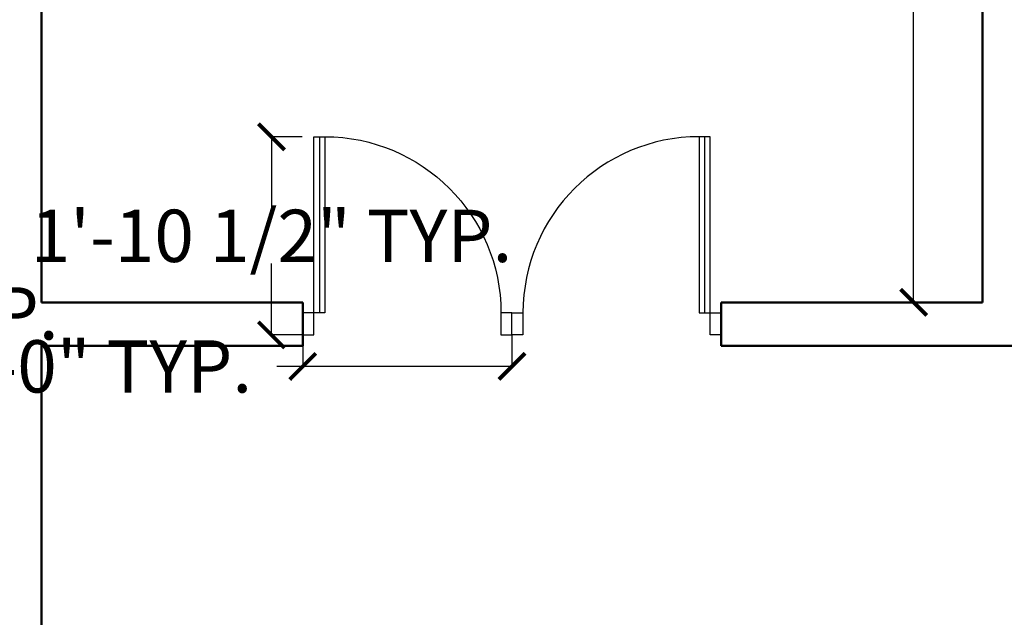
# Model space of a CAD drawing. Units: inches. Extents: x 147 to 1638, y 107 to 941.
# Tile 2 of 17: x 356 to 469, y 216 to 284. Entities that reach past the tile are written whole.
import ezdxf

# ---------------------------------------------------------------- set-up
doc = ezdxf.new("R2010")
doc.units = ezdxf.units.IN
doc.header["$MEASUREMENT"] = 0
for name, color, linetype, lineweight in [('A-ANNO-DIMS', 2, 'Continuous', 15), ('A-Door', 150, 'Continuous', 25), ('walls', 7, 'Continuous', 50)]:
    doc.layers.add(name, color=color, linetype=linetype, lineweight=lineweight)
doc.layers.add('A-Glaz', color=92, linetype='Continuous')
doc.layers.add('NT', color=1, linetype='Continuous')
doc.styles.get("Standard").update_dxf_attribs({"font": 'arial.ttf'})
doc.dimstyles.get("Standard").update_dxf_attribs({"dimtxt": 6, "dimasz": 3, "dimexe": 0.18, "dimexo": 0.0625, "dimgap": 0.09, "dimtad": 0, "dimtih": 1, "dimtoh": 1, "dimdec": 1, "dimzin": 0, "dimdsep": 46, "dimlunit": 3, "dimtxsty": 'Standard', "dimblk": 'ARCHTICK', "dimcen": 0.09, "dimadec": 0, "dimazin": 0, "dimtfac": 1, "dimtdec": 1, "dimtofl": 0, "dimtmove": 0, "dimatfit": 3, "dimfxl": 1, "dimtolj": 1, "dimtzin": 0, "dimarcsym": 0})

# ---------------------------------------------------------------- blocks, each defined once
blk = doc.blocks.new('A$C087A3AA9')
at = {"layer": 'A-Door'}
for points in [[(852.6, 94.7), (852.6, 852.6), (805.3, 852.6), (805.3, 94.7)], [(47.4, 94.7), (47.4, 0), (0, 0), (0, 94.7)], [(900, 94.7), (900, 0), (852.6, 0), (852.6, 94.7)]]:
    blk.add_lwpolyline(points, close=True, dxfattribs=at)
at = {"layer": 'A-Glaz'}
blk.add_line((828.9, 852.6), (828.9, 94.7), dxfattribs=at)
at = {"layer": 'NT'}
blk.add_arc((805.3, 94.7), 757.9, 90, 180, dxfattribs=at)
blk = doc.blocks.new('_ArchTick')
at = {"color": 0, "linetype": 'ByBlock', "const_width": 0.15}
blk.add_lwpolyline([(-0.5, -0.5), (0.5, 0.5)], dxfattribs=at)
blk = doc.blocks.new('*D30')
at = {"layer": 'A-ANNO-DIMS', "color": 0, "lineweight": -2, "transparency": 16777216}
for p, q in [((460.3, 395.72), (458.86, 395.72)), ((459.04, 395.72), (459.04, 326.82)), ((459.04, 251.72), (459.04, 320.62)), ((460.3, 251.72), (458.86, 251.72))]:
    blk.add_line(p, q, dxfattribs=at)
at = {"layer": 'Defpoints', "color": 0, "lineweight": -2, "transparency": 16777216}
for p in [(460.36, 395.72), (459.04, 251.72), (460.36, 251.72)]:
    blk.add_point(p, dxfattribs=at)
at = {"layer": 'A-ANNO-DIMS', "color": 0, "lineweight": -2, "transparency": 16777216, "xscale": 3, "yscale": 3, "zscale": 3}
for p, rotation in [((459.04, 395.72), 90), ((459.04, 251.72), 270)]:
    blk.add_blockref('_ArchTick', p, dxfattribs=dict(at, rotation=rotation))
at = {"layer": 'A-ANNO-DIMS', "color": 0, "transparency": 16777216, "insert": (459.04, 323.72), "char_height": 6, "attachment_point": 5}
blk.add_mtext("\\A1;12'", dxfattribs=at)
blk = doc.blocks.new('*D98')
at = {"layer": 'A-ANNO-DIMS', "color": 0, "lineweight": -2, "transparency": 16777216}
for p, q in [((388.94, 247.92), (388.94, 244.2)), ((412.94, 247.92), (412.94, 244.2)), ((388.94, 244.38), (385.94, 244.38)), ((412.94, 244.38), (388.94, 244.38))]:
    blk.add_line(p, q, dxfattribs=at)
at = {"layer": 'Defpoints', "color": 0, "lineweight": -2, "transparency": 16777216}
for p in [(388.94, 247.98), (412.94, 247.98), (388.94, 244.38)]:
    blk.add_point(p, dxfattribs=at)
at = {"layer": 'A-ANNO-DIMS', "color": 0, "lineweight": -2, "transparency": 16777216, "xscale": 3, "yscale": 3, "zscale": 3, "rotation": 180}
blk.add_blockref('_ArchTick', (388.94, 244.38), dxfattribs=at)
at = {"layer": 'A-ANNO-DIMS', "color": 0, "lineweight": -2, "transparency": 16777216, "xscale": 3, "yscale": 3, "zscale": 3}
blk.add_blockref('_ArchTick', (412.94, 244.38), dxfattribs=at)
at = {"layer": 'A-ANNO-DIMS', "color": 0, "transparency": 16777216, "insert": (338.48, 244.38), "char_height": 6, "attachment_point": 5}
blk.add_mtext('\\A1;SWING DOOR 2\'-0" TYP.', dxfattribs=at)
blk = doc.blocks.new('*D99')
at = {"layer": 'A-ANNO-DIMS', "color": 0, "lineweight": -2, "transparency": 16777216}
for p, q in [((388.88, 270.72), (385.16, 270.72)), ((385.34, 270.72), (385.34, 262.54)), ((385.34, 247.98), (385.34, 256.16)), ((388.88, 247.98), (385.16, 247.98))]:
    blk.add_line(p, q, dxfattribs=at)
at = {"layer": 'Defpoints', "color": 0, "lineweight": -2, "transparency": 16777216}
for p in [(385.34, 270.72), (388.94, 270.72), (388.94, 247.98)]:
    blk.add_point(p, dxfattribs=at)
at = {"layer": 'A-ANNO-DIMS', "color": 0, "lineweight": -2, "transparency": 16777216, "xscale": 3, "yscale": 3, "zscale": 3}
for p, rotation in [((385.34, 270.72), 90), ((385.34, 247.98), 270)]:
    blk.add_blockref('_ArchTick', p, dxfattribs=dict(at, rotation=rotation))
at = {"layer": 'A-ANNO-DIMS', "color": 0, "transparency": 16777216, "insert": (385.34, 259.35), "char_height": 6, "attachment_point": 5}
blk.add_mtext('\\A1;1\'-10 1/2" TYP.', dxfattribs=at)
blk = doc.blocks.new('*D111')
at = {"layer": 'A-ANNO-DIMS', "color": 0, "lineweight": -2, "transparency": 16777216}
for p, q in [((323.17, 280.75), (335.72, 280.75)), ((335.54, 280.75), (335.54, 253.66)), ((335.54, 220.18), (335.54, 247.27)), ((323.17, 220.18), (335.72, 220.18))]:
    blk.add_line(p, q, dxfattribs=at)
at = {"layer": 'Defpoints', "color": 0, "lineweight": -2, "transparency": 16777216}
for p in [(323.11, 280.75), (323.11, 220.18), (335.54, 220.18)]:
    blk.add_point(p, dxfattribs=at)
at = {"layer": 'A-ANNO-DIMS', "color": 0, "lineweight": -2, "transparency": 16777216, "xscale": 3, "yscale": 3, "zscale": 3}
for p, rotation in [((335.54, 280.75), 90), ((335.54, 220.18), 270)]:
    blk.add_blockref('_ArchTick', p, dxfattribs=dict(at, rotation=rotation))
at = {"layer": 'A-ANNO-DIMS', "color": 0, "transparency": 16777216, "insert": (335.54, 250.46), "char_height": 6, "attachment_point": 5}
blk.add_mtext('\\A1;5\'-0 1/2" TYP.', dxfattribs=at)

msp = doc.modelspace()

# ---------------------------------------------------------------- linework, layer by layer
at = {"layer": 'walls'}
for p, q in [((358.94, 395.72), (358.94, 251.72)), ((466.94, 395.72), (466.94, 251.72)), ((358.94, 251.72), (388.94, 251.72)), ((388.94, 246.72), (388.94, 251.72)), ((436.94, 246.72), (436.94, 251.72)), ((436.94, 251.72), (466.94, 251.72)), ((358.94, 246.72), (388.94, 246.72)), ((358.94, 246.72), (358.94, 201.72)), ((436.94, 246.72), (466.94, 246.72)), ((466.94, 246.72), (495.94, 246.72))]:
    msp.add_line(p, q, dxfattribs=at)

# ---------------------------------------------------------------- block references
at = {"layer": 'A-Door', "yscale": 0.0266666667542921, "zscale": 0.0266666667542921}
for xscale in [-0.0266666667542921, 0.0266666667542921]:
    msp.add_blockref('A$C087A3AA9', (412.94, 247.98), dxfattribs=dict(at, xscale=xscale))

# ---------------------------------------------------------------- dimensions: what is measured, and where the dimension line sits
at = {"layer": 'A-ANNO-DIMS'}
dim = msp.add_linear_dim(base=(459.04, 251.72), p1=(460.36, 395.72), p2=(460.36, 251.72), angle=90, dimstyle='Standard', override={"dimclrd": 0, "dimclre": 0, "dimclrt": 0}, dxfattribs=at)
dim.commit()
dim.dimension.update_dxf_attribs({"geometry": '*D30', "text_midpoint": (459.04, 323.72)})
for base, p1, p2, angle, text, picture, middle in [((335.54, 220.18), (323.11, 280.75), (323.11, 220.18), 270, '<> TYP.', '*D111', (335.54, 250.46)), ((385.34, 270.72), (388.94, 247.98), (388.94, 270.72), 90, '<> TYP.', '*D99', (385.34, 259.35)), ((388.94, 244.38), (412.94, 247.98), (388.94, 247.98), 180, 'SWING DOOR <> TYP.', '*D98', (338.48, 244.38))]:
    dim = msp.add_linear_dim(base=base, p1=p1, p2=p2, angle=angle, text=text, dimstyle='Standard', override={"dimdec": 1, "dimlfac": 1, "dimrnd": 0, "dimzin": 1, "dimdsep": 46, "dimlunit": 4, "dimfrac": 2}, dxfattribs=at)
    dim.commit()
    dim.dimension.update_dxf_attribs({"geometry": picture, "text_midpoint": middle})

doc.saveas('drawing.dxf')
